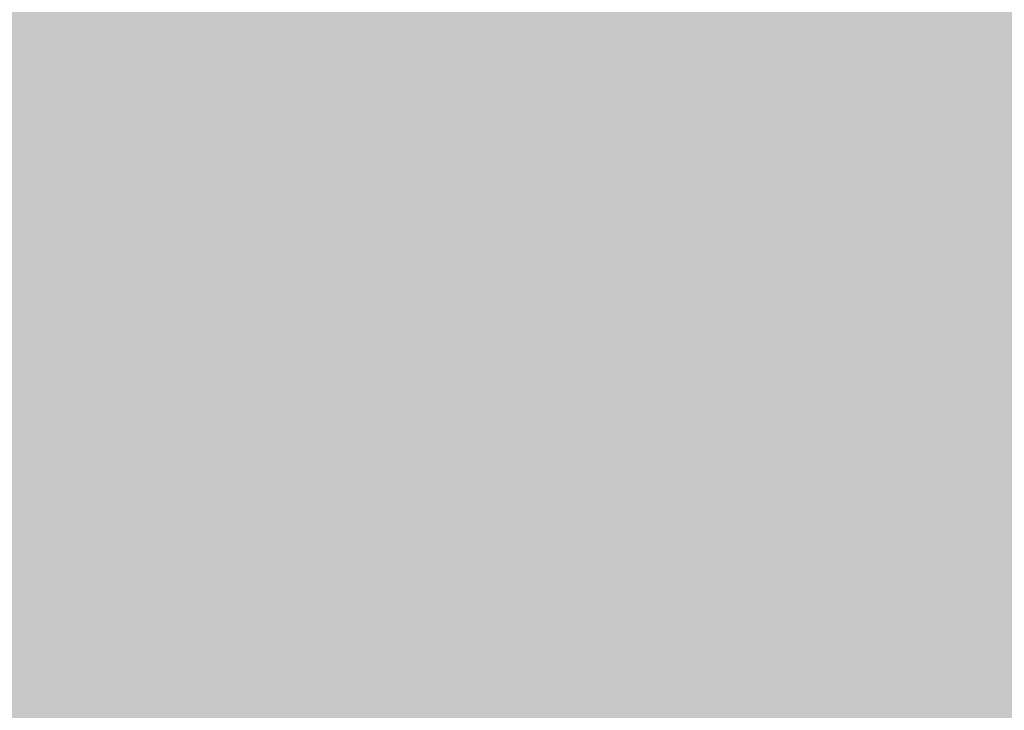
# Model space of a CAD drawing. Units: inches. Extents: x 2091 to 2899, y 967 to 2217.
# Tile 233 of 256: x 2203.4104 to 2203.7172, y 1152.4622 to 1152.6774. Entities that reach past the tile are written whole.
import ezdxf

# ---------------------------------------------------------------- set-up
doc = ezdxf.new("R2010")
doc.units = ezdxf.units.IN
doc.layers.add('A-WALL-PATT', color=141, linetype='Continuous', lineweight=13, true_color=0xadddf7)

msp = doc.modelspace()

# ---------------------------------------------------------------- hatches: boundary and pattern name
at = {"layer": 'A-WALL-PATT'}
h = msp.add_hatch(color=256, dxfattribs=at)
h.dxf.hatch_style = 1
h.paths.add_polyline_path([(2803.1436, 2050.91906), (2203.1436, 2050.91906), (2203.1436, 1090.91906), (2803.1436, 1090.91906)])
h.paths.add_polyline_path([(2635.79885, 1147.54046), (2674.52405, 1147.54046, 0.376086), (2678.52967, 1152.8802), (2678.52967, 1159.55647, 0.333335), (2674.52432, 1163.56185), (2674.52432, 1163.56185), (2674.52432, 1192.93439), (2635.80597, 1192.93439), (2597.08762, 1192.93439), (2597.08762, 1163.56185, 0.333335), (2593.08228, 1159.55647), (2593.08228, 1152.8802, 0.376086), (2597.08789, 1147.54046)], flags=0)
h.paths.add_polyline_path([(2436.01043, 1278.24078, 0.000483), (2435.95264, 1278.21503, -0.001328), (2435.93563, 1278.11169, -0.001711), (2436.11644, 1278.04076, 0.002185)], flags=0)
h.paths.add_polyline_path([(2794.1436, 1143.41906), (2794.1436, 1347.41906), (2543.37017, 1347.41906), (2543.37017, 1351.91906), (2794.1436, 1351.91906), (2794.1436, 1392.71355), (2793.9474, 1392.71355), (2793.9474, 1473.5369), (2794.1436, 1473.5369), (2794.1436, 1531.91906), (2650.1436, 1531.91906), (2650.1436, 1536.41906), (2794.1436, 1536.41906), (2794.1436, 1692.41906), (2609.37561, 1692.41906), (2609.37561, 1644.41906), (2604.87561, 1644.41906), (2604.87561, 1744.91906), (2609.37561, 1744.91906), (2609.37561, 1696.91906), (2794.1436, 1696.91906), (2794.1436, 1780.91906), (2609.6436, 1780.91906), (2493.87561, 1780.91906), (2493.87561, 1785.41906), (2609.6436, 1785.41906), (2794.1436, 1785.41906), (2794.1436, 1847.93882), (2793.95122, 1847.93882), (2793.95122, 1928.76217), (2794.1436, 1928.76217), (2794.1436, 1941.41906), (2614.1436, 1941.41906), (2614.1436, 1821.41906), (2609.6436, 1821.41906), (2609.6436, 1941.41906), (2392.1436, 1941.41906), (2392.1436, 1819.91906), (2387.6436, 1819.91906), (2387.6436, 1941.41906), (2212.1436, 1941.41906), (2212.1436, 1783.91906), (2392.1436, 1783.91906), (2392.1436, 1780.91906), (2212.1436, 1780.91906), (2212.1436, 1629.41906), (2387.6436, 1629.41906), (2387.6436, 1744.91906), (2392.1436, 1744.91906), (2392.1436, 1627.91906), (2317.1436, 1627.91906), (2317.1436, 1551.41906), (2317.1436, 1536.41906), (2459.38359, 1536.41906), (2459.38359, 1602.39648), (2463.88359, 1602.39648), (2463.88359, 1531.91906), (2456.6436, 1531.91906), (2456.6436, 1529.91906), (2452.1436, 1529.91906), (2452.1436, 1531.91906), (2312.6436, 1531.91906), (2312.6436, 1551.41906), (2306.1436, 1551.41906), (2306.1436, 1555.91906), (2308.1436, 1555.91906), (2308.1436, 1551.41906), (2312.6436, 1551.41906), (2312.6436, 1627.91906), (2212.1436, 1627.91906), (2212.1436, 1555.91906), (2270.1436, 1555.91906), (2270.1436, 1551.41906), (2212.1436, 1551.41906), (2212.1436, 1351.91906), (2272.1436, 1351.91906), (2272.1436, 1347.41906), (2212.1436, 1347.41906), (2212.1436, 1275.41906), (2308.1436, 1275.41906), (2308.1436, 1351.91906), (2452.1436, 1351.91906), (2452.1436, 1493.91906), (2456.6436, 1493.91906), (2456.6436, 1347.41906), (2312.6436, 1347.41906), (2312.6436, 1270.91906), (2212.1436, 1270.91906), (2212.1436, 1099.91906), (2281.23752, 1099.91906), (2282.87104, 1110.9138), (2282.00834, 1116.9966), (2278.55774, 1121.4204), (2268.20564, 1128.0562), (2272.08764, 1128.0562), (2273.81294, 1131.927), (2279.42034, 1134.6919), (2285.02784, 1135.2449), (2287.61584, 1137.4568), (2288.04714, 1138.0098), (2289.34114, 1140.7747), (2291.06654, 1139.6687), (2292.36054, 1135.2449), (2295.37984, 1136.9038), (2296.24254, 1135.7979), (2297.10524, 1133.033), (2300.12464, 1138.0098), (2303.14394, 1138.0098), (2304.43794, 1135.7979), (2303.14394, 1133.586), (2306.59464, 1134.6919), (2307.88874, 1133.033), (2310.90804, 1135.2449), (2313.92744, 1134.1389), (2315.62686, 1132.4271), (2308.32004, 1117.5496), (2290.20384, 1109.8079), (2288.90984, 1103.1721), (2289.27231, 1099.91906), (2434.91823, 1099.91906), (2431.59323, 1124.78806), (2429.93023, 1169.55306), (2430.92718, 1240.51969), (2435.65893, 1238.18613), (2437.13523, 1196.55406), (2438.79823, 1143.97306), (2442.67823, 1111.99806), (2446.55823, 1099.91906), (2794.1436, 1099.91906), (2794.1436, 1138.91906), (2548.03245, 1138.91906), (2548.03245, 1143.41906), (2548.03245, 1148.81906), (2546.66846, 1148.03156), (2528.68569, 1179.17862, 0.256256), (2512.03245, 1148.81906), (2512.03245, 1143.41906), (2512.03245, 1138.91906), (2507.53245, 1138.91906), (2507.53245, 1143.41906), (2507.53245, 1148.81906, 0.256256), (2490.8792, 1179.17862), (2472.89644, 1148.03156), (2471.53245, 1148.81906), (2471.53245, 1143.41906), (2467.03245, 1143.41906), (2467.03245, 1269.94579, 0.039061), (2460.90999, 1273.58006), (2467.03245, 1273.58006), (2467.03245, 1286.32536, 0.014511), (2465.21619, 1286.76191), (2467.03245, 1287.05258), (2467.03245, 1323.41906), (2471.53245, 1323.41906), (2471.53245, 1148.81906), (2489.53245, 1179.99597), (2490.89644, 1179.20847), (2490.8792, 1179.17862, -0.256256), (2507.53245, 1148.81906), (2507.53245, 1143.41906), (2512.03245, 1143.41906), (2512.03245, 1148.81906, -0.256256), (2528.68569, 1179.17862), (2528.66846, 1179.20847), (2530.03245, 1179.99597), (2548.03245, 1148.81906), (2548.03245, 1143.41906)], flags=16)
h.paths.add_polyline_path([(2607.76855, 1200.94508), (2607.76855, 1265.03063), (2597.08762, 1281.05201), (2619.78459, 1281.05201), (2627.79528, 1337.12686), (2635.79885, 1337.12686), (2643.81666, 1337.12686), (2651.82736, 1281.05201), (2674.52432, 1281.05201), (2663.8434, 1265.03063), (2663.8434, 1200.94508), (2635.80597, 1200.94508)], flags=0)
edge = h.paths.add_edge_path(flags=0)
edge.add_ellipse((13303.89622, 1272.99872), major_axis=(-10595.31304, 0), ratio=0.84230387009, start_angle=0.628237219, end_angle=0.6465541, ccw=False)
edge.add_ellipse((2711.70045, 1156.85268), major_axis=(2.21977, 0), ratio=0.8423039, start_angle=111.53524, end_angle=180.62824, ccw=False)
edge.add_ellipse((13303.15629, 1272.99872), major_axis=(-10593.02631, 0), ratio=0.84230386954, start_angle=0.528271472, end_angle=0.646554097, ccw=False)
edge.add_line((2710.7646, 1175.3333), (2710.12999, 1175.3333))
edge.add_ellipse((2710.12999, 1176.57978), major_axis=(1.47985, 0), ratio=0.8423039, start_angle=180, end_angle=270, ccw=False)
edge.add_line((2708.65014, 1176.57978), (2708.65014, 1200.78291))
edge.add_ellipse((2710.12999, 1200.78291), major_axis=(1.47985, 0), ratio=0.8423039, start_angle=90, end_angle=180, ccw=False)
edge.add_line((2710.12999, 1202.02939), (2710.46508, 1202.02939))
edge.add_ellipse((13303.15629, 1272.99872), major_axis=(-10593.02631, 0), ratio=0.84230386954, start_angle=-0.090229089, end_angle=0.383866779, ccw=False)
edge.add_ellipse((2710.12999, 1290.92703), major_axis=(-1.47985, 0), ratio=0.8423039, start_angle=0, end_angle=90, ccw=False)
edge.add_line((2708.65014, 1290.92703), (2708.65014, 1315.13017))
edge.add_ellipse((2710.12999, 1315.13017), major_axis=(-1.47985, 0), ratio=0.8423039, start_angle=-90, end_angle=0, ccw=False)
edge.add_line((2710.12999, 1316.37665), (2710.70631, 1316.37665))
edge.add_ellipse((3238.40172, 1296.28957), major_axis=(528.234, 0), ratio=0.84230387, start_angle=176.3495724, end_angle=177.8200497, ccw=False)
edge.add_ellipse((2775.06304, 1071.4507), major_axis=(313.30776, 0), ratio=0.84230387, start_angle=102.1259656, end_angle=103.780529, ccw=False)
edge.add_ellipse((2775.06304, 1078.3057), major_axis=(-305.30289, 0), ratio=0.84230387, start_angle=-79.790461, end_angle=-77.5553727, ccw=False)
edge.add_ellipse((2695.14177, 1541.97538), major_axis=(-250.96022, 0), ratio=0.84230387, start_angle=99.256566, end_angle=102.5549326)
edge.add_line((2741.41033, 1334.21426), (2747.13255, 1337.37848))
edge.add_ellipse((2747.53862, 1336.85748), major_axis=(-0.73992, 0), ratio=0.842304, start_angle=270, end_angle=307.93313, ccw=False)
edge.add_ellipse((2747.53862, 1336.85748), major_axis=(-0.73992, 0), ratio=0.842304, start_angle=232.06687, end_angle=270, ccw=False)
edge.add_line((2747.94469, 1337.37848), (2753.66691, 1334.21426))
edge.add_ellipse((2799.93547, 1541.97538), major_axis=(250.96022, 0), ratio=0.84230387, start_angle=257.4450674, end_angle=260.743434)
edge.add_ellipse((2720.01419, 1078.3057), major_axis=(305.30289, 0), ratio=0.84230387, start_angle=77.5553727, end_angle=79.790461, ccw=False)
edge.add_ellipse((2720.01419, 1071.4507), major_axis=(-313.30776, 0), ratio=0.84230387, start_angle=256.219471, end_angle=257.8740344, ccw=False)
edge.add_ellipse((2256.67551, 1296.28957), major_axis=(-528.234, 0), ratio=0.84230387, start_angle=182.1799503, end_angle=183.6504276, ccw=False)
edge.add_line((2784.37092, 1316.37665), (2784.94725, 1316.37665))
edge.add_ellipse((2784.94725, 1315.13017), major_axis=(1.47985, 0), ratio=0.8423039, start_angle=0, end_angle=90, ccw=False)
edge.add_line((2786.42709, 1315.13017), (2786.42709, 1290.92703))
edge.add_ellipse((2784.94725, 1290.92703), major_axis=(1.47985, 0), ratio=0.8423039, start_angle=270, end_angle=360, ccw=False)
edge.add_ellipse((-7808.07906, 1272.99872), major_axis=(10593.02631, 0), ratio=0.84230386954, start_angle=-0.383866779, end_angle=0.090229089, ccw=False)
edge.add_line((2784.61216, 1202.02939), (2784.94725, 1202.02939))
edge.add_ellipse((2784.94725, 1200.78291), major_axis=(1.47985, 0), ratio=0.8423039, start_angle=0, end_angle=90, ccw=False)
edge.add_line((2786.42709, 1200.78291), (2786.42709, 1176.57978))
edge.add_ellipse((2784.94725, 1176.57978), major_axis=(-1.47985, 0), ratio=0.8423039, start_angle=90, end_angle=180, ccw=False)
edge.add_line((2784.94725, 1175.3333), (2784.31264, 1175.3333))
edge.add_ellipse((-7808.07906, 1272.99872), major_axis=(10593.02631, 0), ratio=0.84230386954, start_angle=-0.618643196, end_angle=-0.528271472, ccw=False)
edge.add_ellipse((2783.37678, 1156.85268), major_axis=(-2.21977, 0), ratio=0.8423039, start_angle=179.37176, end_angle=248.46476, ccw=False)
edge.add_ellipse((-7808.81898, 1272.99872), major_axis=(-10595.31304, 0), ratio=0.84230386576, start_angle=179.353445923, end_angle=179.371762803, ccw=False)
edge.add_ellipse((2780.2973, 1153.50079), major_axis=(-5.24643, 0), ratio=0.8423039, start_angle=90, end_angle=179.35345, ccw=False)
edge.add_line((2780.2973, 1149.08171), (2714.77993, 1149.08171))
edge.add_ellipse((2714.77993, 1153.50079), major_axis=(5.24643, 0), ratio=0.8423039, start_angle=180.64655, end_angle=270, ccw=False)
edge = h.paths.add_edge_path(flags=0)
edge.add_line((2718.18737, 1151.00783), (2718.18737, 1170.47236))
edge.add_ellipse((2721.14706, 1170.47236), major_axis=(-2.95969, 0), ratio=0.8423039, start_angle=-90, end_angle=0, ccw=False)
edge.add_line((2721.14706, 1172.96532), (2773.93017, 1172.96532))
edge.add_ellipse((2773.93017, 1170.47236), major_axis=(-2.95969, 0), ratio=0.8423039, start_angle=180, end_angle=270, ccw=False)
edge.add_line((2776.88987, 1170.47236), (2776.88987, 1151.00783))
edge.add_line((2776.88987, 1151.00783), (2718.18737, 1151.00783))
edge = h.paths.add_edge_path(flags=0)
edge.add_line((2718.18737, 1180.23415), (2718.18737, 1199.05783))
edge.add_ellipse((2747.53862, 1320.39864), major_axis=(147.01792, 0), ratio=0.84230387, start_angle=256.4018653, end_angle=283.5981347)
edge.add_line((2776.88987, 1199.05783), (2776.88987, 1180.23415))
edge.add_ellipse((2747.53862, 1301.57496), major_axis=(147.01792, 0), ratio=0.84230387, start_angle=256.4018653, end_angle=283.5981347, ccw=False)
edge = h.paths.add_edge_path(flags=0)
edge.add_ellipse((13303.15629, 1272.99872), major_axis=(-10591.54646, 0), ratio=0.84230386955, start_angle=0.055594314, end_angle=0.377764194, ccw=False)
edge.add_line((2711.61686, 1262.72171), (2715.66741, 1249.4954))
edge.add_ellipse((6413.89196, 1241.69192), major_axis=(-3698.23616, 0), ratio=0.8423038695, start_angle=-0.12089737, end_angle=0.36407635)
edge.add_line((2715.76104, 1218.19245), (2711.93431, 1203.16736))
edge = h.paths.add_edge_path(flags=0)
edge.add_line((2718.18737, 1251.07457), (2716.00249, 1267.45044))
edge.add_ellipse((2742.15117, 1202.18954), major_axis=(81.77258, 0), ratio=0.84230387, start_angle=94.277421, end_angle=111.8349538, ccw=False)
edge.add_line((2737.00975, 1270.93063), (2758.06748, 1270.93063))
edge.add_ellipse((2752.92606, 1202.18954), major_axis=(81.77258, 0), ratio=0.84230387, start_angle=68.1650462, end_angle=85.722579, ccw=False)
edge.add_line((2779.07475, 1267.45044), (2776.88987, 1251.07457))
edge.add_ellipse((2750.33806, 1187.88536), major_axis=(79.57966, 0), ratio=0.84230387, start_angle=67.2080851, end_angle=85.1299304)
edge.add_line((2756.03466, 1254.74366), (2739.04258, 1254.74366))
edge.add_ellipse((2744.73917, 1187.88536), major_axis=(79.57966, 0), ratio=0.84230387, start_angle=94.8700696, end_angle=112.7919149)
edge = h.paths.add_edge_path(flags=0)
edge.add_line((2783.14293, 1203.16736), (2779.31619, 1218.19245))
edge.add_ellipse((-918.81473, 1241.69192), major_axis=(3698.23616, 0), ratio=0.8423038695, start_angle=-0.36407635, end_angle=0.12089737)
edge.add_line((2779.40983, 1249.4954), (2783.46037, 1262.72171))
edge.add_ellipse((-7808.07906, 1272.99872), major_axis=(-10591.54646, 0), ratio=0.84230386954, start_angle=179.622235806, end_angle=179.944405687, ccw=False)
edge = h.paths.add_edge_path(flags=0)
edge.add_ellipse((2734.20089, 1286.69044), major_axis=(-0.35661, 6.34008), ratio=0.6038336, start_angle=89.002014, end_angle=253.657408, ccw=False)
edge.add_line((2730.369, 1286.54181), (2730.369, 1301.35198))
edge.add_line((2730.369, 1301.35198), (2735.91331, 1305.2148))
edge.add_ellipse((2736.38492, 1304.73456), major_axis=(0.73992, 0), ratio=0.842304, start_angle=90, end_angle=134.48021, ccw=False)
edge.add_line((2736.38492, 1305.3578), (2738.03278, 1305.3578))
edge.add_line((2738.03278, 1305.3578), (2738.03278, 1307.70793))
edge.add_ellipse((2794.20164, 1307.70793), major_axis=(56.16886, 0), ratio=0.84230387, start_angle=150.56143, end_angle=180, ccw=False)
edge.add_ellipse((2700.87559, 1307.70793), major_axis=(-56.16886, 0), ratio=0.84230387, start_angle=180, end_angle=209.43857, ccw=False)
edge.add_line((2757.04445, 1307.70793), (2757.04445, 1305.3578))
edge.add_line((2757.04445, 1305.3578), (2758.69232, 1305.3578))
edge.add_ellipse((2758.69232, 1304.73456), major_axis=(-0.73992, 0), ratio=0.842304, start_angle=225.51979, end_angle=270, ccw=False)
edge.add_line((2759.16392, 1305.2148), (2764.70823, 1301.35198))
edge.add_line((2764.70823, 1301.35198), (2764.70823, 1286.54181))
edge.add_ellipse((2760.87634, 1286.69044), major_axis=(0.35661, 6.34008), ratio=0.6038336, start_angle=106.342592, end_angle=270.997986, ccw=False)
edge.add_line((2757.04445, 1285.79709), (2757.04445, 1307.70793))
edge.add_ellipse((2700.87559, 1307.70793), major_axis=(-56.16886, 0), ratio=0.84230387, start_angle=180, end_angle=209.43857)
edge.add_ellipse((2794.20164, 1307.70793), major_axis=(56.16886, 0), ratio=0.84230387, start_angle=150.56143, end_angle=180)
edge.add_line((2738.03278, 1307.70793), (2738.03278, 1285.79709))
h.paths.add_polyline_path([(2417.81227, 1104.4497), (2413.49227, 1102.5297), (2410.61227, 1103.9697), (2409.17227, 1106.3697), (2407.25227, 1107.3297), (2406.29227, 1109.7297), (2405.33227, 1114.0497), (2405.33227, 1117.8897), (2406.29227, 1120.1297), (2407.25227, 1119.8097), (2408.84832, 1118.32766), (2410.17395, 1119.42417), (2410.21127, 1120.4057), (2411.04073, 1121.41905), (2410.69927, 1119.8587), (2410.17395, 1119.42417), (2410.08845, 1117.17611), (2411.13284, 1116.20632), (2413.97227, 1119.3297), (2416.85227, 1120.7697), (2416.86972, 1120.79878), (2417.03507, 1119.40512), (2417.89621, 1118.14338), (2418.29227, 1118.3697), (2419.54445, 1120.03927), (2419.36092, 1118.38749), (2419.03211, 1119.35615), (2418.39894, 1118.51193), (2419.25227, 1114.5297), (2418.79409, 1107.19879)], flags=0)
h.paths.add_polyline_path([(2508.87017, 1347.41906), (2508.37017, 1347.41906), (2508.37017, 1351.91906), (2508.87017, 1351.91906)], flags=0)
h.paths.add_polyline_path([(2473.37017, 1347.41906), (2472.37017, 1347.41906), (2467.87017, 1347.41906), (2467.87017, 1455.41906), (2472.37017, 1455.41906), (2472.37017, 1352.41906), (2473.37017, 1352.41906)], flags=0)
h.paths.add_polyline_path([(2352.10624, 1217.4462), (2349.22624, 1218.8862), (2347.78624, 1221.2862), (2345.86624, 1222.2462), (2344.90624, 1224.6462), (2343.94624, 1228.9662), (2343.94624, 1232.8062), (2344.90624, 1235.0462), (2345.86624, 1234.7262), (2347.46229, 1233.24415), (2348.78792, 1234.34066), (2348.82524, 1235.3222), (2349.6547, 1236.33555), (2349.31324, 1234.7752), (2348.78792, 1234.34066), (2348.70242, 1232.0926), (2349.74681, 1231.12282), (2352.58624, 1234.2462), (2355.46624, 1235.6862), (2355.48369, 1235.71528), (2355.64904, 1234.32161), (2356.51018, 1233.05988), (2356.90624, 1233.2862), (2358.15842, 1234.95576), (2357.97489, 1233.30398), (2357.64608, 1234.27264), (2357.01291, 1233.42842), (2357.86624, 1229.4462), (2357.40806, 1222.11529), (2356.42624, 1219.3662)], flags=0)
h.paths.add_polyline_path([(2348.2968, 1112.22442), (2347.0138, 1112.31042), (2345.5298, 1114.12742), (2345.7318, 1115.85842), (2346.8118, 1116.98242), (2346.8118, 1114.64642), (2345.8668, 1114.21442), (2346.8798, 1114.30042)], flags=0)
h.paths.add_polyline_path([(2347.0138, 1110.92642), (2346.2718, 1110.49342), (2346.6098, 1111.18642)], flags=0)
h.paths.add_polyline_path([(2345.8668, 1118.19442), (2345.5298, 1117.32942), (2343.7078, 1118.02142), (2344.3828, 1118.62642)], flags=0)
h.paths.add_polyline_path([(2346.6768, 1109.28242), (2346.0698, 1108.07142), (2345.8668, 1110.06142)], flags=0)
h.paths.add_polyline_path([(2345.0568, 1119.75142), (2343.6398, 1119.75142), (2343.9778, 1121.13542)], flags=0)
h.paths.add_polyline_path([(2345.2598, 1116.55042), (2345.1248, 1115.85842), (2344.9218, 1115.68542), (2344.7198, 1116.37742)], flags=0)
h.paths.add_polyline_path([(2345.6648, 1112.31042), (2345.4618, 1111.53242), (2344.0448, 1111.96442), (2344.6518, 1112.57042)], flags=0)
h.paths.add_polyline_path([(2345.1918, 1113.34942), (2344.4498, 1113.86842), (2344.7198, 1114.38742)], flags=0)
h.paths.add_polyline_path([(2344.6518, 1116.80942), (2344.1798, 1115.68542), (2344.6518, 1115.33942), (2343.9098, 1114.90642), (2343.0328, 1115.94442), (2343.6398, 1116.46342)], flags=0)
h.paths.add_polyline_path([(2345.8668, 1106.68642), (2344.9898, 1105.56242), (2344.5168, 1106.60042)], flags=0)
h.paths.add_polyline_path([(2344.8548, 1110.06142), (2344.5168, 1109.28242), (2344.1128, 1109.71542)], flags=0)
h.paths.add_polyline_path([(2344.0448, 1113.52242), (2343.4378, 1113.08942), (2342.7628, 1113.95442)], flags=0)
h.paths.add_polyline_path([(2344.3148, 1111.01242), (2342.9648, 1110.32042), (2342.9648, 1111.09942)], flags=0)
h.paths.add_polyline_path([(2345.1248, 1104.69742), (2344.5848, 1103.74542), (2344.4498, 1104.26442)], flags=0)
h.paths.add_polyline_path([(2342.8298, 1121.22242), (2341.7498, 1120.53042), (2340.5358, 1121.04942), (2340.1308, 1121.82842), (2340.6708, 1122.95242), (2341.1428, 1121.82842), (2341.6148, 1122.00142)], flags=0)
h.paths.add_polyline_path([(2342.9648, 1119.75142), (2343.0328, 1118.45342), (2342.0878, 1118.02142), (2342.0198, 1119.49142)], flags=0)
h.paths.add_polyline_path([(2342.6948, 1116.89642), (2341.9528, 1116.63642), (2342.0198, 1117.32942)], flags=0)
h.paths.add_polyline_path([(2343.0328, 1112.22442), (2342.0198, 1111.79142), (2341.5478, 1112.22442), (2342.3578, 1113.34942)], flags=0)
h.paths.add_polyline_path([(2343.7748, 1104.43742), (2342.6278, 1102.88042), (2342.6948, 1104.61042), (2343.4378, 1105.12942)], flags=0)
h.paths.add_polyline_path([(2342.0198, 1115.07942), (2340.8058, 1115.51242), (2340.9408, 1116.37742)], flags=0)
h.paths.add_polyline_path([(2341.4808, 1120.09742), (2341.4808, 1119.40542), (2341.0758, 1119.57842), (2341.1428, 1120.09742)], flags=0)
h.paths.add_polyline_path([(2341.8178, 1114.47342), (2340.9408, 1113.08942), (2340.8058, 1114.56042)], flags=0)
h.paths.add_polyline_path([(2341.1428, 1118.54042), (2340.9408, 1116.98242), (2339.0508, 1117.67542), (2339.0508, 1118.62642)], flags=0)
h.paths.add_polyline_path([(2342.6948, 1101.66842), (2341.9528, 1101.84142), (2342.5598, 1102.36142)], flags=0)
h.paths.add_polyline_path([(2340.3328, 1119.66542), (2338.4438, 1119.57842), (2337.9038, 1120.35742), (2339.6578, 1120.61642)], flags=0)
h.paths.add_polyline_path([(2340.3328, 1115.33942), (2340.0628, 1113.69542), (2339.3878, 1115.33942)], flags=0)
h.paths.add_polyline_path([(2341.8178, 1103.83142), (2341.5478, 1102.88042), (2341.1428, 1103.65842)], flags=0)
h.paths.add_polyline_path([(2339.0508, 1122.86642), (2337.2958, 1121.82842), (2337.0938, 1123.12542), (2337.7688, 1123.81842)], flags=0)
h.paths.add_polyline_path([(2339.1178, 1121.74142), (2338.8478, 1121.22242), (2338.1738, 1121.04942), (2338.3758, 1121.56842)], flags=0)
h.paths.add_polyline_path([(2339.1858, 1119.31942), (2338.6458, 1118.71342), (2338.2408, 1118.10742), (2338.2408, 1118.88642)], flags=0)
h.paths.add_polyline_path([(2341.1428, 1101.92842), (2340.6028, 1101.23642), (2340.0628, 1101.84142), (2340.6028, 1102.36142)], flags=0)
h.paths.add_polyline_path([(2337.6338, 1117.76142), (2336.6208, 1118.28042), (2337.2958, 1118.97242)], flags=0)
h.paths.add_polyline_path([(2336.8238, 1119.57842), (2334.7988, 1118.97242), (2335.2038, 1120.35742), (2336.5538, 1120.87642)], flags=0)
h.paths.add_polyline_path([(2339.1178, 1100.45742), (2337.3638, 1100.54342), (2336.7558, 1101.23642)], flags=0)
h.paths.add_polyline_path([(2336.3508, 1122.43342), (2336.0138, 1121.91442), (2334.9338, 1122.43342), (2334.5288, 1123.47142), (2335.7438, 1122.77942)], flags=0)
h.paths.add_polyline_path([(2334.7318, 1120.87642), (2334.2588, 1120.35742), (2334.0568, 1120.78942), (2334.5968, 1121.30842)], flags=0)
h.paths.add_polyline_path([(2334.4618, 1122.17442), (2332.5718, 1121.30842), (2331.3568, 1122.17442), (2332.0998, 1122.86642)], flags=0)
h.paths.add_polyline_path([(2334.2588, 1118.54042), (2333.3818, 1118.45342), (2333.6518, 1119.31942)], flags=0)
h.paths.add_polyline_path([(2335.5418, 1102.27442), (2334.1918, 1102.62042), (2335.2718, 1103.31242)], flags=0)
h.paths.add_polyline_path([(2332.7068, 1119.66542), (2331.6948, 1120.44342), (2332.5048, 1120.78942)], flags=0)
h.paths.add_polyline_path([(2334.7318, 1101.14942), (2333.5168, 1101.58242), (2333.9888, 1101.75542)], flags=0)
h.paths.add_polyline_path([(2332.6398, 1116.63642), (2331.0868, 1116.29042), (2331.9648, 1118.19442)], flags=0)
h.paths.add_polyline_path([(2330.7498, 1121.56842), (2330.2768, 1120.27042), (2328.5228, 1119.31942), (2328.9948, 1121.04942)], flags=0)
h.paths.add_polyline_path([(2330.7498, 1118.62642), (2330.0078, 1117.50242), (2329.8728, 1118.02142)], flags=0)
h.paths.add_polyline_path([(2332.0998, 1102.36142), (2330.5468, 1102.01442), (2331.6948, 1102.96642)], flags=0)
h.paths.add_polyline_path([(2329.5348, 1113.60842), (2329.0628, 1112.31042), (2328.5898, 1113.34942)], flags=0)
h.paths.add_polyline_path([(2328.3878, 1117.84842), (2327.5098, 1116.55042), (2327.1728, 1117.76142)], flags=0)
h.paths.add_polyline_path([(2329.7378, 1106.51342), (2329.5348, 1105.30242), (2328.2528, 1106.08142)], flags=0)
h.paths.add_polyline_path([(2328.6578, 1114.38742), (2328.0498, 1114.12742), (2328.3198, 1114.90642)], flags=0)
h.paths.add_polyline_path([(2328.3198, 1112.22442), (2327.1058, 1112.13742), (2326.7008, 1112.65642)], flags=0)
h.paths.add_polyline_path([(2326.9028, 1115.25242), (2326.7008, 1114.12742), (2325.2158, 1113.60842), (2326.0928, 1115.33942)], flags=0)
h.paths.add_polyline_path([(2326.6328, 1108.33042), (2326.0928, 1107.37942), (2325.8908, 1108.50342), (2326.4978, 1109.10942)], flags=0)
h.paths.add_polyline_path([(2615.1436, 1531.91906), (2609.6436, 1531.91906), (2609.6436, 1620.41906), (2614.1436, 1620.41906), (2614.1436, 1536.41906), (2615.1436, 1536.41906)], flags=0)
h.paths.add_polyline_path([(2545.1436, 1563.41906), (2464.1436, 1563.41906), (2464.1436, 1632.41906), (2509.1436, 1632.41906), (2509.1436, 1627.91906), (2509.1436, 1603.91906), (2468.6436, 1603.91906), (2468.6436, 1567.91906), (2540.6436, 1567.91906), (2540.6436, 1591.91906), (2545.1436, 1591.91906)], flags=0)
h.paths.add_polyline_path([(2388.96905, 1549.98573), (2357.43418, 1549.98573), (2357.43418, 1623.36078), (2399.36278, 1623.36078), (2435.68947, 1623.36078), (2435.59255, 1602.55927), (2435.59255, 1602.39648), (2388.96905, 1602.39648)], flags=0)
h.paths.add_polyline_path([(2388.88063, 1555.80915), (2374.90443, 1555.80915), (2374.90443, 1600.57156), (2374.90443, 1615.45765), (2406.35088, 1615.45765), (2406.35088, 1618.93943), (2412.17429, 1615.45765), (2406.35088, 1611.97586), (2406.35088, 1615.45765), (2388.88063, 1615.45765)], flags=0)
h.paths.add_polyline_path([(2568.87561, 1644.41906), (2453.37561, 1644.41906), (2453.37561, 1785.41906), (2457.87561, 1785.41906), (2457.87561, 1648.91906), (2568.87561, 1648.91906)], flags=0)
h.paths.add_polyline_path([(2212.1436, 1945.91906), (2212.1436, 2041.91906), (2794.1436, 2041.91906), (2794.1436, 1945.91906)], flags=16)
h.paths.add_polyline_path([(2271.08273, 1964.31724), (2776.85297, 1964.31724), (2776.85297, 2037.16962), (2271.08273, 2037.16962)], flags=8)
h.paths.add_polyline_path([(2380.64929, 1536.82414), (2461.04081, 1536.82414), (2461.04081, 1554.65259), (2380.64929, 1554.65259)], flags=8)
h.paths.add_polyline_path([(2240.75571, 1609.72545), (2309.18583, 1609.72545), (2309.18583, 1617.6982), (2240.75571, 1617.6982)], flags=8)
h.paths.add_polyline_path([(2212.67726, 1313.5041), (2282.59152, 1313.5041), (2282.59152, 1322.74524), (2212.67726, 1322.74524)], flags=8)
h.paths.add_polyline_path([(2457.11198, 1114.77857), (2558.48158, 1114.77857), (2558.48158, 1142.21968), (2457.11198, 1142.21968)], flags=8)
h.paths.add_polyline_path([(2473.44234, 1273.01007), (2604.64123, 1273.01007), (2604.64123, 1318.34693), (2473.44234, 1318.34693)], flags=8)
h.paths.add_polyline_path([(2638.8763, 1626.97743), (2684.25037, 1627.97674), (2684.03848, 1637.59749), (2638.66442, 1636.59819)], flags=8)
h.paths.add_polyline_path([(2537.59055, 1453.79345), (2628.38955, 1453.79345), (2628.38955, 1475.34481), (2537.59055, 1475.34481)], flags=8)
h.paths.add_polyline_path([(2504.13764, 1714.6324), (2554.64719, 1714.6324), (2554.64719, 1730.23771), (2504.13764, 1730.23771)], flags=8)
h.paths.add_polyline_path([(2487.50118, 1575.65187), (2535.09712, 1575.65187), (2535.09712, 1598.37765), (2487.50118, 1598.37765)], flags=8)
h.paths.add_polyline_path([(2709.0994, 1735.71028), (2740.0166, 1735.71028), (2740.0166, 1749.93764), (2709.0994, 1749.93764)], flags=8)
h.paths.add_polyline_path([(2442.43842, 1792.17166), (2564.72884, 1792.17166), (2564.72884, 1842.00016), (2442.43842, 1842.00016)], flags=8)
h.paths.add_polyline_path([(2655.8158, 1809.64408), (2789.52014, 1806.6938), (2790.08498, 1832.29164), (2656.38064, 1835.24192)], flags=8)
h.paths.add_polyline_path([(2234.8427, 1797.72014), (2368.59285, 1794.76885), (2369.16072, 1820.50413), (2235.41056, 1823.45542)], flags=8)
h.paths.add_polyline_path([(2245.13847, 1644.00633), (2398.42773, 1640.6239), (2398.99484, 1666.32482), (2245.70557, 1669.70725)], flags=8)
h.paths.add_polyline_path([(2306.14285, 1431.16852), (2413.76831, 1428.79369), (2414.33315, 1454.39153), (2306.70768, 1456.76636)], flags=8)
h.paths.add_polyline_path([(2306.83458, 1458.23314), (2393.38048, 1456.32345), (2393.93281, 1481.35436), (2307.38691, 1483.26405)], flags=8)

doc.saveas('drawing.dxf')
